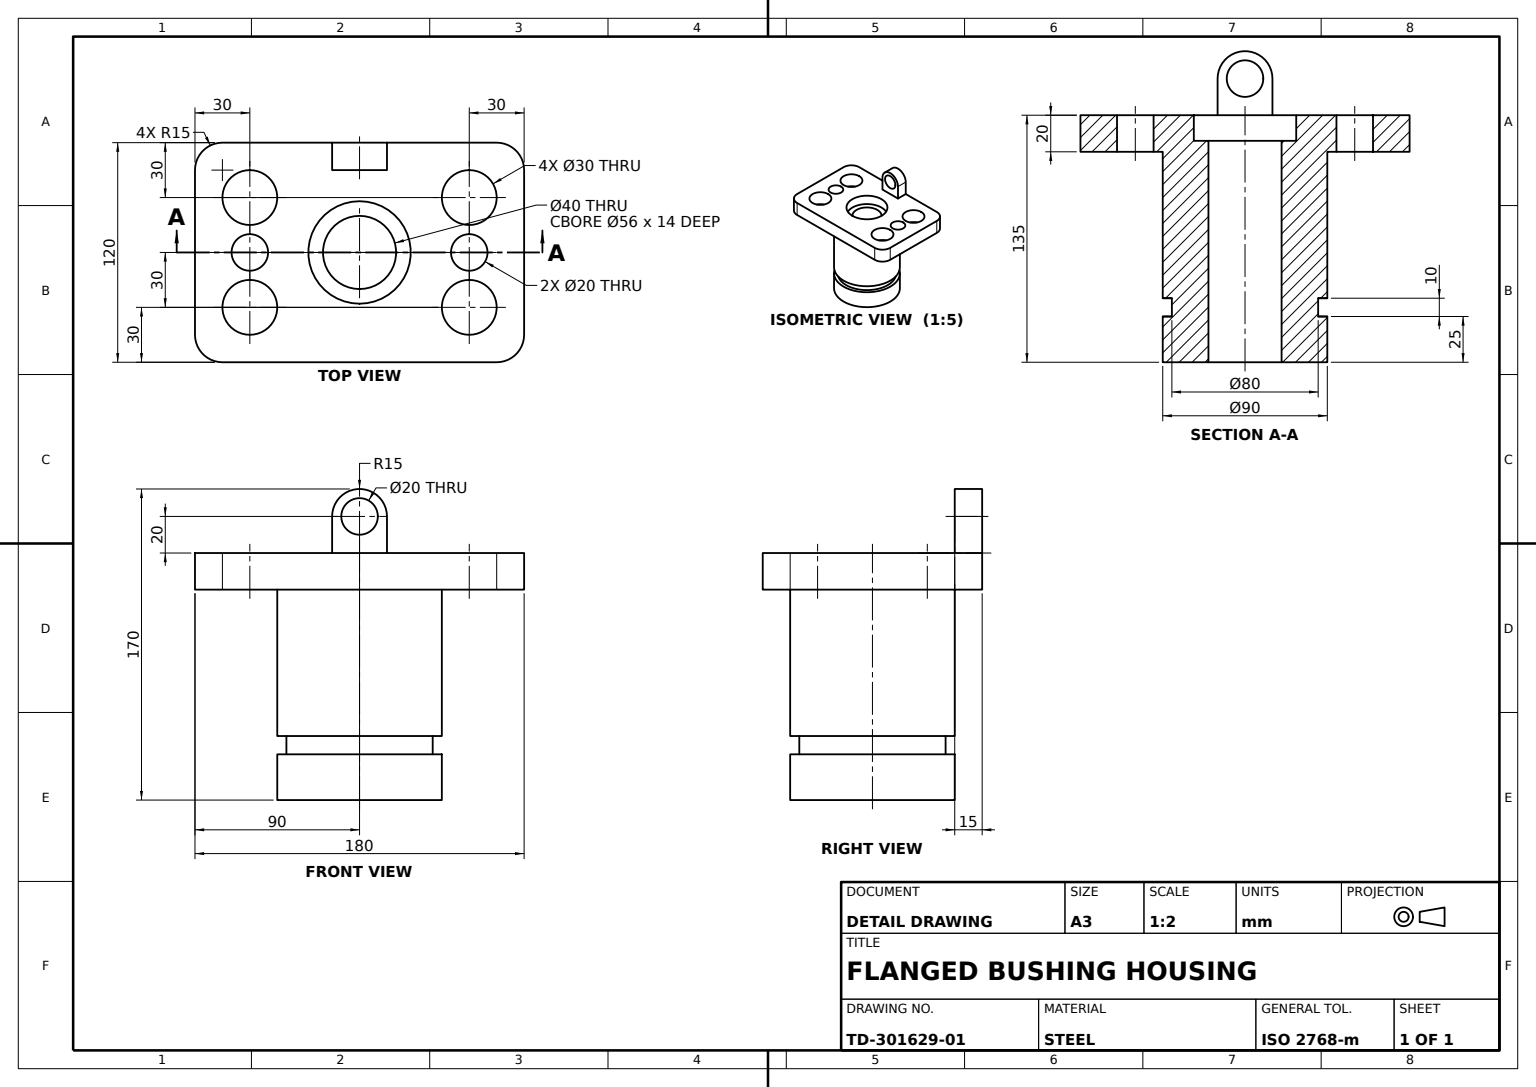
SolidWorks part; units mm, degrees
material "Plain Carbon Steel"
ref_plane "Front Plane" through (0, 0, 0) normal (0, 0, 1) x (1, 0, 0)
ref_plane "Top Plane" through (0, 0, 0) normal (0, 1, 0) x (1, 0, 0)
ref_plane "Right Plane" through (0, 0, 0) normal (1, 0, 0) x (0, 0, -1)
sketch "Bushing Profile Sketch" plane through (0, 0, 0) normal (0, 0, 1) x (1, 0, 0)
  line L3 (45, 0) -> (45, -100)
  line L4 (45, -100) -> (40, -100)
  line L5 (40, -100) -> (40, -110)
  line L6 (40, -110) -> (45, -110)
  line L7 (45, -110) -> (45, -135)
  line L8 (45, -135) -> (20, -135)
  line L9 (0, -88.6363) -> (0, 0) construction
  line L10 (20, -14) -> (20, -135)
  line L11 (20, -14) -> (28, -14)
  line L12 (28, -14) -> (28, 0)
  line L13 (28, 0) -> (45, 0)
  dimension "D1" = 5
  dimension "D2" = 20
  dimension "D3" = 10
  dimension "D4" = 25
  dimension "D5" = 25
  dimension "D6" = 135
  dimension "D7" = 121
  dimension "D8" = 28
revolve "Bushing Body" add sketch "Bushing Profile Sketch" angle 360 about L9
sketch "Flange Plate Sketch" plane through (0, 0, 0) normal (0, 1, 0) x (1, 0, 0)
  line L0 (-60, -30) -> (-60, 30) construction
  line L1 (-75, -60) -> (75, -60)
  line L2 (-90, -45) -> (-90, 45)
  line L3 (-75, 60) -> (75, 60)
  line L4 (90, -45) -> (90, 45)
  line L5 (-90, -60) -> (90, 60) construction
  line L6 (-90, 60) -> (90, -60) construction
  line L7 (0, 0) -> (0, 70.8095) construction
  arc A0 (-75, -60) -> (-90, -45) centre (-75, -45) cw
  arc A1 (75, -60) -> (90, -45) centre (75, -45) ccw
  arc A2 (75, 60) -> (90, 45) centre (75, 45) cw
  arc A3 (-90, 45) -> (-75, 60) centre (-75, 45) cw
  circle A4 centre (-60, -30) radius 15
  circle A5 centre (-60, 0) radius 10
  circle A6 centre (-60, 30) radius 15
  circle A7 centre (60, -30) radius 15
  circle A8 centre (60, 0) radius 10
  circle A9 centre (60, 30) radius 15
  circle A10 centre (0, 0) radius 45 construction
  circle A11 centre (0, 0) radius 45
  point P0 (0, 0)
  dimension "D3" = 15
  dimension "D4" = 30
  dimension "D7" = 20
  dimension "D8" = 30
  dimension "D1" = 120
  dimension "D2" = 180
  dimension "D5" = 30
  dimension "D6" = 30
  dimension "D9" = 30
extrude "Flange Plate 120x180" add sketch "Flange Plate Sketch" against normal blind 20
sketch "Eyelet Lug Sketch" plane through (0, 0, -60) normal (0, 0, -1) x (-1, 0, 0)
  line L0 (-15, 20) -> (-15, 0)
  line L1 (-75, 0) -> (75, 0) construction
  line L2 (-15, 0) -> (15, 0)
  line L3 (15, 0) -> (15, 20)
  arc A0 (15, 20) -> (-15, 20) centre (0, 20) ccw
  circle A1 centre (0, 20) radius 10
  dimension "D1" = 15
  dimension "D2" = 20
  dimension "D3" = 20
extrude "Eyelet Lug" add sketch "Eyelet Lug Sketch" against normal blind 15
